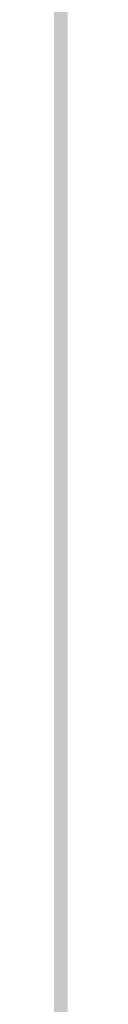
# Model space of a CAD drawing. Units: inches. Extents: x 2083 to 3317, y 1141 to 2115.
# Tile 192 of 256: x 3126.9582 to 3126.9594, y 1263.3548 to 1263.6134. Entities that reach past the tile are written whole.
import ezdxf

# ---------------------------------------------------------------- set-up
doc = ezdxf.new("R2010")
doc.units = ezdxf.units.IN
doc.layers.add('A-ANNO-DIMS', color=2, linetype='Continuous', lineweight=18)
doc.layers.add('A-WALL-PATT', color=251, linetype='Continuous', lineweight=13, true_color=0x636466)
doc.styles.get("Standard").update_dxf_attribs({"font": 'arial.ttf'})
doc.dimstyles.new('ISO-25', dxfattribs={"dimtxt": 12, "dimasz": 12, "dimexe": 1.25, "dimexo": 0.625, "dimtad": 1, "dimlunit": 3, "dimtxsty": 'Standard', "dimcen": 2.5, "dimadec": 0, "dimazin": 0, "dimtfac": 1, "dimtmove": 0, "dimatfit": 3, "dimfxl": 1, "dimarcsym": 0})

# ---------------------------------------------------------------- blocks, each defined once
blk = doc.blocks.new('*D26')
at = {"layer": 'A-ANNO-DIMS', "color": 0, "lineweight": -2, "transparency": 16777216}
for p, q in [((3088.98584, 1274.91509), (3088.98584, 1270.95196)), ((3111.24004, 1274.91509), (3111.24004, 1270.95196)), ((3076.98584, 1272.20196), (2840.26245, 1272.20196)), ((3111.24004, 1272.20196), (3088.98584, 1272.20196)), ((3123.24004, 1272.20196), (3135.24004, 1272.20196))]:
    blk.add_line(p, q, dxfattribs=at)
at = {"layer": 'A-ANNO-DIMS', "color": 0, "transparency": 16777216}
for points in [[(3076.98584, 1274.20196), (3076.98584, 1270.20196), (3088.98584, 1272.20196)], [(3123.24004, 1274.20196), (3123.24004, 1270.20196), (3111.24004, 1272.20196)]]:
    blk.add_solid(points, dxfattribs=at)
at = {"layer": 'Defpoints', "color": 0, "transparency": 16777216}
for p in [(3088.98584, 1275.54009), (3111.24004, 1275.54009), (3088.98584, 1272.20196)]:
    blk.add_point(p, dxfattribs=at)
at = {"layer": 'A-ANNO-DIMS', "color": 0, "transparency": 16777216, "insert": (2952.62415, 1279.0316), "char_height": 12, "attachment_point": 5}
blk.add_mtext('NIGHTSTAND 1\'-10 1/2" TYP.', dxfattribs=at)
blk = doc.blocks.new('*D27')
at = {"layer": 'A-ANNO-DIMS', "color": 0, "lineweight": -2, "transparency": 16777216}
for p, q in [((3114.57817, 1309.79428), (3114.57817, 1321.79428)), ((3111.86504, 1297.79428), (3115.82817, 1297.79428)), ((3114.57817, 1297.79428), (3114.57817, 1275.54009)), ((3111.86504, 1275.54009), (3115.82817, 1275.54009)), ((3114.57817, 1263.54009), (3114.57817, 1140.98859))]:
    blk.add_line(p, q, dxfattribs=at)
at = {"layer": 'A-ANNO-DIMS', "color": 0, "transparency": 16777216}
for points in [[(3112.57817, 1309.79428), (3116.57817, 1309.79428), (3114.57817, 1297.79428)], [(3112.57817, 1263.54009), (3116.57817, 1263.54009), (3114.57817, 1275.54009)]]:
    blk.add_solid(points, dxfattribs=at)
at = {"layer": 'Defpoints', "color": 0, "transparency": 16777216}
for p in [(3111.24004, 1297.79428), (3111.24004, 1275.54009), (3114.57817, 1275.54009)]:
    blk.add_point(p, dxfattribs=at)
at = {"layer": 'A-ANNO-DIMS', "color": 0, "transparency": 16777216, "insert": (3107.74853, 1196.26434), "char_height": 12, "attachment_point": 5, "rotation": 90}
blk.add_mtext('1\'-10 1/2" TYP.', dxfattribs=at)

msp = doc.modelspace()

# ---------------------------------------------------------------- hatches: boundary and pattern name
at = {"layer": 'A-WALL-PATT'}
h = msp.add_hatch(color=256, dxfattribs=at)
h.dxf.hatch_style = 1
h.paths.add_polyline_path([(3126.95978, 2020.76136), (2748.95978, 2020.76136), (2604.95978, 2020.76136), (2226.95978, 2020.76136), (2226.95978, 1702.76136), (2466.95978, 1702.76136), (2466.95978, 1582.76136), (2418.95978, 1582.76136), (2418.95978, 1477.76136), (2226.95978, 1477.76136), (2226.95978, 1263.26136), (2544.95978, 1263.26136), (2544.95978, 1411.76136), (2604.95978, 1411.76136), (2685.95978, 1411.76136), (2685.95978, 1420.76136), (2604.95978, 1420.76136), (2604.95978, 1573.76136), (2604.95978, 1702.76136), (2604.95978, 2011.76136), (2748.95978, 2011.76136), (2748.95978, 1702.76136), (2862.95978, 1702.76136), (2862.95978, 1621.76136), (2871.95978, 1621.76136), (2871.95978, 1702.76136), (2883.95978, 1702.76136), (2883.95978, 1706.93946, -0.026459), (2883.95978, 1711.76136), (2757.95978, 1711.76136), (2757.95978, 1807.76136), (2787.95978, 1807.76136), (2787.95978, 1812.26136), (2757.95978, 1812.26136), (2757.95978, 2011.76136), (2877.95978, 2011.76136), (2877.95978, 1812.26136), (2847.95978, 1812.26136), (2847.95978, 1807.76136), (2889.83574, 1807.76136), (2889.83574, 1812.26136), (2882.45978, 1812.26136), (2882.45978, 2011.76136), (3117.95978, 2011.76136), (3117.95978, 1812.26136), (2937.83574, 1812.26136), (2937.83574, 1807.76136), (2995.70978, 1807.76136), (2995.70978, 1796.11767), (3000.20978, 1796.11767), (3000.20978, 1807.76136), (3117.95978, 1807.76136), (3117.95978, 1711.76136), (3000.20978, 1711.76136), (3000.20978, 1760.11767), (2998.5727, 1760.11767, -0.020711), (2995.70978, 1760.11767), (2995.70978, 1711.76136), (2931.95978, 1711.76136), (2931.95978, 1702.76136), (3126.95978, 1702.76136)])
h.paths.add_polyline_path([(2471.45978, 2011.76136), (2471.45978, 1810.01136), (2462.71694, 1810.01136), (2462.71694, 1805.51136), (2505.95978, 1805.51136), (2505.95978, 1810.01136), (2475.95978, 1810.01136), (2475.95978, 2011.76136), (2595.95978, 2011.76136), (2595.95978, 1810.01136), (2565.95978, 1810.01136), (2565.95978, 1805.51136), (2595.95978, 1805.51136), (2595.95978, 1711.76136), (2235.95978, 1711.76136), (2235.95978, 1805.51136), (2353.70978, 1805.51136), (2353.70978, 1796.05416), (2358.20978, 1796.05416), (2358.20978, 1805.51136), (2414.71694, 1805.51136), (2414.71694, 1810.01136), (2235.95978, 1810.01136), (2235.95978, 2011.76136)], flags=16)
h.paths.add_polyline_path([(2270.20473, 1994.61001), (2270.20473, 1970.61001), (2246.20473, 1970.61001), (2246.20473, 1994.61001)], flags=0)
edge = h.paths.add_edge_path(flags=0)
edge.add_ellipse((2332.02739, 1899.79818), major_axis=(-3.04299, 3.04299), ratio=0.1682525, start_angle=-161.33217, end_angle=-156.30711, ccw=False)
edge.add_ellipse((2333.08204, 1898.74353), major_axis=(-1.05465, 1.05465), ratio=0.4535321, start_angle=-123.37102, end_angle=-94.15911)
edge = h.paths.add_edge_path(flags=0)
edge.add_ellipse((2332.02739, 1968.87629), major_axis=(3.04299, 3.04299), ratio=0.1682525, start_angle=18.66783, end_angle=23.69289)
edge.add_spline(control_points=[(2332.9256, 1970.6911), (2332.22677, 1970.3361), (2330.89371, 1969.65891), (2328.41308, 1970.93214), (2327.20393, 1967.74871), (2324.7096, 1969.95559), (2322.53282, 1967.01235), (2320.01285, 1971.29581), (2317.68031, 1968.15784), (2316.04053, 1967.10205), (2315.4269, 1966.8096)], knot_values=[0, 0, 0, 0, 2.267059, 4.324559, 6.685584, 8.878641, 11.121502, 14.300359, 17.755284, 19.732645, 19.732645, 19.732645, 19.732645], degree=3, periodic=0)
edge.add_ellipse((2332.02739, 1968.87629), major_axis=(3.04299, 3.04299), ratio=0.1682525, start_angle=18.66783, end_angle=23.69289, ccw=False)
edge.add_ellipse((2333.08204, 1969.93094), major_axis=(1.05465, 1.05465), ratio=0.4535321, start_angle=56.62898, end_angle=85.84089, ccw=False)
edge = h.paths.add_edge_path(flags=0)
edge.add_spline(control_points=[(2296.42829, 1967.98791), (2293.6278, 1965.33631), (2287.70362, 1959.72709), (2299.74386, 1949.9957), (2294.53259, 1935.66853), (2290.57323, 1920.60351), (2293.39412, 1909.97369), (2296.18541, 1904.96654)], knot_values=[0.099185, 0.099185, 0.099185, 0.099185, 0.345301, 0.619822, 0.982653, 1.386093, 1.810555, 1.810555, 1.810555, 1.810555], degree=3, periodic=0)
edge.add_spline(control_points=[(2296.18541, 1904.96654), (2297.38358, 1902.6193), (2298.00097, 1901.94931), (2298.55297, 1901.46815)], knot_values=[0.006246, 0.006246, 0.006246, 0.006246, 0.055476, 0.055476, 0.055476, 0.055476], degree=3, periodic=0)
edge.add_spline(control_points=[(2298.55297, 1901.46815), (2297.25861, 1900.92322), (2295.22529, 1900.23213), (2293.06023, 1900.61421), (2292.10142, 1900.78841), (2292.08958, 1900.79057)], knot_values=[0.312835, 0.312835, 0.312835, 0.312835, 0.40178, 0.474987, 0.475903, 0.475903, 0.475903, 0.475903], degree=3, periodic=0)
edge.add_arc((2292.79365, 1904.66411), 3.93701, 215.4209, 259.69818, ccw=False)
edge.add_spline(control_points=[(2289.58531, 1902.3823), (2289.47665, 1902.53509), (2289.36848, 1902.68804), (2289.26086, 1902.84117)], knot_values=[0.102872, 0.102872, 0.102872, 0.102872, 0.116896, 0.116896, 0.116896, 0.116896], degree=3, periodic=0)
edge.add_spline(control_points=[(2289.26086, 1902.84117), (2288.6866, 1902.55019), (2287.64005, 1902.0199), (2285.88134, 1901.87395), (2283.85297, 1901.50435), (2281.71999, 1899.71054), (2278.46699, 1899.49294), (2276.15714, 1901.8832), (2272.25895, 1899.80407), (2267.77761, 1901.84318), (2262.24388, 1900.18403), (2257.41493, 1901.78206), (2254.31837, 1900.72612), (2253.17828, 1900.33734)], knot_values=[0, 0, 0, 0, 1.907977, 3.477176, 5.261074, 7.972851, 11.680248, 13.717921, 16.939592, 22.789562, 27.502503, 33.595215, 37.145618, 37.145618, 37.145618, 37.145618], degree=3, periodic=0)
edge.add_line((2253.17828, 1900.33734), (2250.24424, 1902.84117))
edge.add_line((2250.24424, 1902.84117), (2250.24424, 1965.8333))
edge.add_line((2250.24424, 1965.8333), (2253.17828, 1968.33712))
edge.add_spline(control_points=[(2253.17828, 1968.33712), (2254.31837, 1967.94835), (2257.41493, 1966.89241), (2262.24388, 1968.49043), (2267.77761, 1966.83128), (2271.52673, 1968.53722), (2273.87591, 1967.82829), (2274.2067, 1967.72764)], knot_values=[0, 0, 0, 0, 0.09018, 0.244935, 0.364644, 0.513233, 0.537855, 0.537855, 0.537855, 0.537855], degree=3, periodic=0)
edge.add_arc((2274.35289, 1963.79335), 3.93701, 72.05113, 92.12795, ccw=False)
edge.add_arc((2281.29693, 1985.23), 18.5963, 252.051134, 288.565722)
edge.add_arc((2292.31672, 1956.02888), 12.64608, 71.026788, 113.778218, ccw=False)
edge = h.paths.add_edge_path(flags=0)
edge.add_spline(control_points=[(2274.89941, 1951.85619), (2275.06616, 1951.61659), (2275.23269, 1951.37659), (2275.39799, 1951.13585)], knot_values=[1.409916, 1.409916, 1.409916, 1.409916, 1.43159, 1.43159, 1.43159, 1.43159], degree=3, periodic=0)
edge.add_spline(control_points=[(2275.39799, 1951.13585), (2275.79211, 1950.56189), (2276.17923, 1949.98377), (2276.54555, 1949.3971)], knot_values=[1.358238, 1.358238, 1.358238, 1.358238, 1.409916, 1.409916, 1.409916, 1.409916], degree=3, periodic=0)
edge.add_line((2276.54555, 1949.3971), (2277.43729, 1947.86218))
edge.add_spline(control_points=[(2277.43729, 1947.86218), (2276.30383, 1945.67311), (2274.6397, 1942.42688), (2274.63161, 1938.0939), (2272.79912, 1930.85155), (2274.35643, 1943.89705), (2275.94768, 1947.92336), (2276.54555, 1949.3971)], knot_values=[0.005632, 0.005632, 0.005632, 0.005632, 0.186014, 0.266002, 0.357087, 0.59639, 0.739732, 0.739732, 0.739732, 0.739732], degree=3, periodic=0)
edge.add_spline(control_points=[(2276.54555, 1949.3971), (2276.17923, 1949.98377), (2275.79211, 1950.56189), (2275.39799, 1951.13585)], knot_values=[1.358238, 1.358238, 1.358238, 1.358238, 1.409916, 1.409916, 1.409916, 1.409916], degree=3, periodic=0)
edge.add_spline(control_points=[(2275.39799, 1951.13585), (2274.9425, 1950.08045), (2274.20776, 1948.02527), (2273.9346, 1944.85148), (2272.46853, 1937.62749), (2273.46622, 1945.69647), (2274.70062, 1951.05947), (2274.89941, 1951.85619)], knot_values=[0.104364, 0.104364, 0.104364, 0.104364, 0.189636, 0.269624, 0.36071, 0.600013, 0.644622, 0.644622, 0.644622, 0.644622], degree=3, periodic=0)
h.paths.add_polyline_path([(2269.16751, 1963.12757, -0.357527), (2268.17063, 1960.97637, -0.092561), (2268.17063, 1939.43632, -0.357527), (2269.16751, 1937.28512, -0.357527), (2267.01631, 1938.282, -0.164785), (2254.68558, 1938.282, -0.357527), (2252.53438, 1937.28512, -0.357527), (2253.53126, 1939.43632, -0.092561), (2253.53126, 1960.97637, -0.357527), (2252.53438, 1963.12757, -0.357527), (2254.68558, 1962.13069, -0.164785), (2267.01631, 1962.13069, -0.357527)], flags=0)
h.paths.add_polyline_path([(2248.87407, 1967.8018), (2248.87407, 1957.02771), (2249.45778, 1957.02771), (2249.45778, 1911.64676), (2248.87407, 1911.64676), (2248.87407, 1900.87267), (2246.51186, 1900.87267, 0.197327), (2244.14966, 1902.45687), (2244.14966, 1966.21759, 0.197327), (2246.51186, 1967.8018)], flags=0)
h.paths.add_polyline_path([(2269.16751, 1931.38934, -0.357527), (2268.17063, 1929.23814, -0.092561), (2268.17063, 1907.6981, -0.357527), (2269.16751, 1905.54689, -0.357527), (2267.01631, 1906.54377, -0.164785), (2254.68558, 1906.54377, -0.357527), (2252.53438, 1905.54689, -0.357527), (2253.53126, 1907.6981, -0.092561), (2253.53126, 1929.23814, -0.357527), (2252.53438, 1931.38934, -0.357527), (2254.68558, 1930.39246, -0.164785), (2267.01631, 1930.39246, -0.357527)], flags=0)
edge = h.paths.add_edge_path(flags=0)
edge.add_spline(control_points=[(2276.19686, 1906.7237), (2276.16814, 1909.02893), (2276.11405, 1913.37185), (2270.59842, 1924.92498), (2273.90517, 1919.01278), (2275.92171, 1916.26206), (2275.47457, 1912.40215), (2277.25787, 1910.38062), (2276.69604, 1908.22504), (2276.64622, 1906.81302), (2276.61782, 1906.00841)], knot_values=[0, 0, 0, 0, 8.61026, 16.221274, 18.843057, 23.804898, 27.440828, 29.356102, 31.203478, 33.650687, 33.650687, 33.650687, 33.650687], degree=3, periodic=0)
edge.add_spline(control_points=[(2276.61782, 1906.00841), (2276.62331, 1905.62414), (2276.49774, 1904.62866), (2275.44178, 1903.85473), (2274.93731, 1903.08045), (2274.85908, 1902.84117)], knot_values=[0.156488, 0.156488, 0.156488, 0.156488, 0.184398, 0.231376, 0.250598, 0.250598, 0.250598, 0.250598], degree=3, periodic=0)
edge.add_line((2274.85908, 1902.84117), (2276.50598, 1902.84117))
edge.add_spline(control_points=[(2276.50598, 1902.84117), (2276.78831, 1903.08494), (2277.66507, 1904.1252), (2278.24954, 1904.34074), (2277.65387, 1908.52739), (2278.15567, 1906.22781), (2278.10046, 1905.28595), (2278.84667, 1904.06901), (2277.85679, 1903.41495), (2277.87419, 1902.99105), (2277.90356, 1902.84117)], knot_values=[0.059574, 0.059574, 0.059574, 0.059574, 0.080753, 0.103741, 0.16972, 0.176036, 0.207137, 0.240474, 0.262341, 0.27366, 0.27366, 0.27366, 0.27366], degree=3, periodic=0)
edge.add_line((2277.90356, 1902.84117), (2280.02983, 1902.84117))
edge.add_spline(control_points=[(2280.02983, 1902.84117), (2279.88822, 1903.0884), (2279.49926, 1903.98155), (2280.15228, 1905.93935), (2278.10362, 1909.65776), (2279.76239, 1907.18529), (2280.3279, 1904.87486), (2280.48511, 1903.48959), (2281.46327, 1903.24943), (2281.75834, 1902.9365), (2281.83404, 1902.84117)], knot_values=[0.013856, 0.013856, 0.013856, 0.013856, 0.034874, 0.088867, 0.107879, 0.126738, 0.158714, 0.193757, 0.217487, 0.226722, 0.226722, 0.226722, 0.226722], degree=3, periodic=0)
edge.add_spline(control_points=[(2281.83404, 1902.84117), (2281.78753, 1902.8267), (2281.64702, 1902.78299), (2281.39553, 1902.85949), (2281.08808, 1902.98524), (2280.72068, 1903.0609), (2280.33345, 1903.02573), (2280.12477, 1902.89888), (2280.02983, 1902.84117)], knot_values=[0, 0, 0, 0, 0.14413, 0.435517, 0.749276, 1.153046, 1.548371, 1.878348, 1.878348, 1.878348, 1.878348], degree=3, periodic=0)
edge.add_line((2280.02983, 1902.84117), (2277.90356, 1902.84117))
edge.add_spline(control_points=[(2277.90356, 1902.84117), (2277.89286, 1902.79586), (2277.8654, 1902.67964), (2277.60748, 1902.68748), (2277.27405, 1902.8007), (2276.83792, 1902.61977), (2276.58381, 1902.78926), (2276.50598, 1902.84117)], knot_values=[0, 0, 0, 0, 0.127189, 0.326199, 0.628009, 1.24357, 1.515331, 1.515331, 1.515331, 1.515331], degree=3, periodic=0)
edge.add_line((2276.50598, 1902.84117), (2274.85908, 1902.84117))
edge.add_spline(control_points=[(2274.85908, 1902.84117), (2274.81444, 1902.89859), (2274.72513, 1903.01345), (2274.49348, 1903.11897), (2274.24429, 1902.96054), (2273.93712, 1903.18494), (2273.61404, 1902.98314), (2273.40832, 1902.88304), (2273.32225, 1902.84117)], knot_values=[0, 0, 0, 0, 0.21843, 0.436957, 0.687977, 0.990379, 1.398396, 1.69185, 1.69185, 1.69185, 1.69185], degree=3, periodic=0)
edge.add_spline(control_points=[(2273.32225, 1902.84117), (2273.61674, 1903.44569), (2274.274, 1904.53825), (2276.02724, 1904.5737), (2276.20696, 1906.58364), (2276.19686, 1906.7237)], knot_values=[0.012227, 0.012227, 0.012227, 0.012227, 0.059472, 0.106218, 0.134458, 0.134458, 0.134458, 0.134458], degree=3, periodic=0)
h.paths.add_polyline_path([(2270.77605, 1897.78983), (2270.77605, 1873.78983), (2246.77605, 1873.78983), (2246.77605, 1897.78983)], flags=0)
h.paths.add_polyline_path([(2353.70978, 1760.00506), (2353.70978, 1760.05416), (2358.20978, 1760.05416, -0.033729)], flags=0)
h.paths.add_polyline_path([(2321.81912, 1737.52919), (2341.99533, 1737.52919, -0.414214), (2343.20327, 1736.32124), (2343.20327, 1721.0206, -0.414214), (2341.99533, 1719.81265), (2321.81912, 1719.81265, -0.414214), (2320.61117, 1721.0206), (2320.61117, 1736.32124, -0.414214)], flags=0)
h.paths.add_polyline_path([(2324.23501, 1736.32124), (2339.57944, 1736.32124, -0.414214), (2341.99533, 1733.90535), (2341.99533, 1725.44973, -0.414214), (2339.57944, 1723.03384), (2333.68059, 1723.03384), (2333.84532, 1722.04547, -0.870646), (2335.4254, 1721.82589, -0.767327), (2333.92269, 1721.42324), (2331.29102, 1721.42324, -0.767327), (2329.78832, 1721.82589, -0.870646), (2331.3684, 1722.04547), (2331.53313, 1723.03384), (2324.23501, 1723.03384, -0.414214), (2321.81912, 1725.44973), (2321.81912, 1733.90535, -0.414214)], flags=0)
h.paths.add_polyline_path([(2570.48379, 1928.61544), (2589.68379, 1928.61544), (2590.16883, 1928.61544), (2590.16883, 1904.9934), (2570.48379, 1904.9934)], flags=0)
h.paths.add_polyline_path([(2574.44732, 1927.26382, -1), (2572.82884, 1927.26382, -1)], flags=0)
h.paths.add_polyline_path([(2573.08987, 1926.94088), (2573.92503, 1927.77604), (2574.14774, 1927.55333), (2573.31258, 1926.71817)], flags=0)
h.paths.add_polyline_path([(2578.77906, 1919.72962, -1), (2571.59166, 1919.72962, -1)], flags=0)
h.paths.add_polyline_path([(2578.38536, 1919.72962, -1), (2571.98536, 1919.72962, -1)], flags=0)
h.paths.add_polyline_path([(2331.59576, 1729.47622, -1), (2333.61795, 1729.47622, -1)], flags=0)
h.paths.add_polyline_path([(2578.03423, 1927.26382, -1), (2576.41574, 1927.26382, -1)], flags=0)
h.paths.add_polyline_path([(2576.68885, 1927.53109), (2576.91156, 1927.7538), (2577.74673, 1926.91863), (2577.52402, 1926.69592)], flags=0)
h.paths.add_polyline_path([(2578.13906, 1909.85954, -1), (2572.23166, 1909.85954, -1)], flags=0)
h.paths.add_polyline_path([(2577.74536, 1909.85954, -1), (2572.62536, 1909.85954, -1)], flags=0)
h.paths.add_polyline_path([(2583.79772, 1927.26382, -1), (2582.17923, 1927.26382, -1)], flags=0)
h.paths.add_polyline_path([(2582.71865, 1927.7538), (2583.55381, 1926.91863), (2583.3311, 1926.69592), (2582.49594, 1927.53109)], flags=0)
h.paths.add_polyline_path([(2582.49594, 1927.53109), (2582.71865, 1927.7538), (2583.55381, 1926.91863), (2583.3311, 1926.69592)], flags=0)
h.paths.add_polyline_path([(2587.73906, 1920.52962, -1), (2581.83166, 1920.52962, -1)], flags=0)
h.paths.add_polyline_path([(2587.34536, 1920.52962, -1), (2582.22536, 1920.52962, -1)], flags=0)
h.paths.add_polyline_path([(2587.38462, 1927.26382, -1), (2585.76613, 1927.26382, -1)], flags=0)
h.paths.add_polyline_path([(2586.08199, 1926.98025), (2586.91716, 1927.81541), (2587.13987, 1927.5927), (2586.3047, 1926.75754)], flags=0)
h.paths.add_polyline_path([(2588.37906, 1910.65954, -1), (2581.19166, 1910.65954, -1)], flags=0)
h.paths.add_polyline_path([(2587.98536, 1910.65954, -1), (2581.58536, 1910.65954, -1)], flags=0)
h.paths.add_polyline_path([(2417.16773, 1729.4779), (2437.34394, 1729.4779, -0.414214), (2438.55188, 1728.26995), (2438.55188, 1712.96931, -0.414214), (2437.34394, 1711.76136), (2417.16773, 1711.76136, -0.414214), (2415.95978, 1712.96931), (2415.95978, 1728.26995, -0.414214)], flags=0)
h.paths.add_polyline_path([(2419.58362, 1728.26995), (2434.92805, 1728.26995, -0.414214), (2437.34394, 1725.85406), (2437.34394, 1717.39844, -0.414214), (2434.92805, 1714.98255), (2429.0292, 1714.98255), (2429.19393, 1713.99418, -0.870646), (2430.77401, 1713.7746, -0.767327), (2429.2713, 1713.37195), (2426.63963, 1713.37195, -0.767327), (2425.13693, 1713.7746, -0.870646), (2426.71701, 1713.99418), (2426.88174, 1714.98255), (2419.58362, 1714.98255, -0.414214), (2417.16773, 1717.39844), (2417.16773, 1725.85406, -0.414214)], flags=0)
h.paths.add_polyline_path([(2419.58362, 1728.26995), (2434.92805, 1728.26995, -0.414214), (2437.34394, 1725.85406), (2437.34394, 1717.39844, -0.414214), (2434.92805, 1714.98255), (2429.0292, 1714.98255), (2428.35812, 1719.00903), (2427.55282, 1719.00903), (2426.88174, 1714.98255), (2419.58362, 1714.98255, -0.414214), (2417.16773, 1717.39844), (2417.16773, 1725.85406, -0.414214)], flags=0)
h.paths.add_polyline_path([(2426.94437, 1721.42492, -1), (2428.96656, 1721.42492, -1)], flags=0)
h.paths.add_polyline_path([(2475.95978, 1702.76136), (2595.95978, 1702.76136), (2595.95978, 1582.76136), (2475.95978, 1582.76136)], flags=16)
h.paths.add_polyline_path([(2427.95978, 1573.76136), (2595.95978, 1573.76136), (2595.95978, 1468.76136), (2595.95978, 1420.76136), (2384.45978, 1420.76136), (2384.45978, 1468.76136), (2427.95978, 1468.76136)], flags=16)
h.paths.add_polyline_path([(2379.95978, 1468.76136), (2379.95978, 1420.76136), (2235.95978, 1420.76136), (2235.95978, 1468.76136)], flags=16)
h.paths.add_polyline_path([(2317.816, 1466.69577), (2337.9922, 1466.69577, -0.414214), (2339.20015, 1465.48782), (2339.20015, 1450.18718, -0.414214), (2337.9922, 1448.97923), (2317.816, 1448.97923, -0.414214), (2316.60805, 1450.18718), (2316.60805, 1465.48782, -0.414214)], flags=0)
h.paths.add_polyline_path([(2320.23189, 1465.48782), (2335.57631, 1465.48782, -0.414214), (2337.9922, 1463.07193), (2337.9922, 1454.61631, -0.414214), (2335.57631, 1452.20042), (2329.67747, 1452.20042), (2329.84219, 1451.21205, -0.870646), (2331.42228, 1450.99247, -0.767327), (2329.91957, 1450.58983), (2327.2879, 1450.58983, -0.767327), (2325.7852, 1450.99247, -0.870646), (2327.36528, 1451.21205), (2327.53001, 1452.20042), (2320.23189, 1452.20042, -0.414214), (2317.816, 1454.61631), (2317.816, 1463.07193, -0.414214)], flags=0)
h.paths.add_polyline_path([(2320.23189, 1465.48782), (2335.57631, 1465.48782, -0.414214), (2337.9922, 1463.07193), (2337.9922, 1454.61631, -0.414214), (2335.57631, 1452.20042), (2329.67747, 1452.20042), (2329.00638, 1456.22691), (2328.20109, 1456.22691), (2327.53001, 1452.20042), (2320.23189, 1452.20042, -0.414214), (2317.816, 1454.61631), (2317.816, 1463.07193, -0.414214)], flags=0)
h.paths.add_polyline_path([(2327.59264, 1458.6428, -1), (2329.61483, 1458.6428, -1)], flags=0)
h.paths.add_polyline_path([(2244.41174, 1433.34045), (2241.92094, 1433.34045, -0.414214), (2240.01786, 1435.24354), (2240.01786, 1440.95281, -0.414211), (2241.92093, 1442.8559), (2244.41174, 1442.8559, -1.976472)], flags=0)
h.paths.add_polyline_path([(2245.35689, 1434.39754, -0.414214), (2245.35689, 1441.79881, -2.144098)], flags=0)
h.paths.add_polyline_path([(2535.95978, 1416.26136), (2535.95978, 1272.26136), (2235.95978, 1272.26136), (2235.95978, 1416.26136)], flags=16)
h.paths.add_polyline_path([(2260.11956, 1384.29284), (2260.11956, 1362.03865), (2237.86537, 1362.03865), (2237.86537, 1384.29284)], flags=0)
edge = h.paths.add_edge_path(flags=0)
edge.add_line((2318.25185, 1362.0933), (2318.1458, 1362.00097))
edge.add_ellipse((2317.44512, 1360.43104), major_axis=(2.82164, 2.82164), ratio=0.1682525, start_angle=18.66783, end_angle=20.94813, ccw=False)
edge.add_ellipse((2318.42305, 1361.40897), major_axis=(0.97793, 0.97793), ratio=0.4535321, start_angle=56.62898, end_angle=70.2262, ccw=False)
edge = h.paths.add_edge_path(flags=0)
edge.add_line((2319.10737, 1295.57108), (2319.01504, 1295.67713))
edge.add_ellipse((2317.44512, 1296.37781), major_axis=(-2.82164, 2.82164), ratio=0.1682525, start_angle=-161.33217, end_angle=-159.05187, ccw=False)
edge.add_ellipse((2318.42305, 1295.39988), major_axis=(-0.97793, 0.97793), ratio=0.4535321, start_angle=-123.37102, end_angle=-109.7738)
edge = h.paths.add_edge_path(flags=0)
edge.add_spline(control_points=[(2284.21035, 1301.17022), (2284.58069, 1300.44472), (2284.89119, 1299.89202), (2285.15955, 1299.46102)], knot_values=[0.039066, 0.039066, 0.039066, 0.039066, 0.055476, 0.055476, 0.055476, 0.055476], degree=3, periodic=0)
edge.add_line((2285.15955, 1299.46102), (2284.21035, 1301.17022))
edge = h.paths.add_edge_path(flags=0)
edge.add_line((2280.41246, 1297.29801), (2283.36999, 1297.03612))
edge.add_line((2283.36999, 1297.03612), (2286.40569, 1297.92631))
edge.add_spline(control_points=[(2286.40569, 1297.92631), (2285.30549, 1297.46312), (2284.34478, 1297.12915), (2283.36999, 1297.03612)], knot_values=[0.394369, 0.394369, 0.394369, 0.394369, 0.475903, 0.475903, 0.475903, 0.475903], degree=3, periodic=0)
edge.add_spline(control_points=[(2283.36999, 1297.03612), (2283.28139, 1297.02767), (2282.31629, 1296.95734), (2281.3125, 1297.13448), (2280.42344, 1297.29602), (2280.41246, 1297.29801)], knot_values=[0.312835, 0.312835, 0.312835, 0.312835, 0.320246, 0.393453, 0.394369, 0.394369, 0.394369, 0.394369], degree=3, periodic=0)
edge = h.paths.add_edge_path(flags=0)
edge.add_line((2284.43556, 1359.60729), (2280.44629, 1355.32805))
edge.add_line((2280.44629, 1355.32805), (2279.57999, 1351.01775))
edge.add_line((2279.57999, 1351.01775), (2282.41297, 1346.58043))
edge.add_spline(control_points=[(2282.41297, 1346.58043), (2283.15333, 1345.58924), (2284.2529, 1344.0289), (2284.80104, 1342.38717), (2284.93516, 1341.80554)], knot_values=[1.240098, 1.240098, 1.240098, 1.240098, 1.332892, 1.382712, 1.382712, 1.382712, 1.382712], degree=3, periodic=0)
edge.add_spline(control_points=[(2284.93516, 1341.80554), (2285.31911, 1340.1406), (2285.23303, 1338.4092), (2284.90994, 1336.65412)], knot_values=[1.097484, 1.097484, 1.097484, 1.097484, 1.240098, 1.240098, 1.240098, 1.240098], degree=3, periodic=0)
edge.add_spline(control_points=[(2284.90994, 1336.65412), (2284.58685, 1334.89904), (2284.02675, 1333.12027), (2283.46264, 1331.36058)], knot_values=[0.95487, 0.95487, 0.95487, 0.95487, 1.097484, 1.097484, 1.097484, 1.097484], degree=3, periodic=0)
edge.add_line((2283.46264, 1331.36058), (2281.89038, 1326.15336))
edge.add_line((2281.89038, 1326.15336), (2280.75626, 1321.05609))
edge.add_line((2280.75626, 1321.05609), (2280.2992, 1316.00198))
edge.add_line((2280.2992, 1316.00198), (2280.71593, 1310.95007))
edge.add_line((2280.71593, 1310.95007), (2282.02809, 1305.97214))
edge.add_line((2282.02809, 1305.97214), (2284.21035, 1301.17022))
edge.add_spline(control_points=[(2284.21035, 1301.17022), (2283.34073, 1302.73019), (2282.6119, 1304.33649), (2282.02809, 1305.97214)], knot_values=[0.099185, 0.099185, 0.099185, 0.099185, 0.241799, 0.241799, 0.241799, 0.241799], degree=3, periodic=0)
edge.add_spline(control_points=[(2282.02809, 1305.97214), (2281.44428, 1307.60778), (2281.00549, 1309.27276), (2280.71593, 1310.95007)], knot_values=[0.241799, 0.241799, 0.241799, 0.241799, 0.384413, 0.384413, 0.384413, 0.384413], degree=3, periodic=0)
edge.add_spline(control_points=[(2280.71593, 1310.95007), (2280.43324, 1312.58761), (2280.28939, 1314.27696), (2280.29889, 1315.96203), (2280.2992, 1316.00198)], knot_values=[0.384413, 0.384413, 0.384413, 0.384413, 0.523647, 0.527028, 0.527028, 0.527028, 0.527028], degree=3, periodic=0)
edge.add_spline(control_points=[(2280.2992, 1316.00198), (2280.31233, 1317.68696), (2280.47787, 1319.36793), (2280.75626, 1321.05609)], knot_values=[0.527028, 0.527028, 0.527028, 0.527028, 0.669642, 0.669642, 0.669642, 0.669642], degree=3, periodic=0)
edge.add_spline(control_points=[(2280.75626, 1321.05609), (2281.03465, 1322.74425), (2281.42588, 1324.43961), (2281.89038, 1326.15336)], knot_values=[0.669642, 0.669642, 0.669642, 0.669642, 0.812256, 0.812256, 0.812256, 0.812256], degree=3, periodic=0)
edge.add_spline(control_points=[(2281.89038, 1326.15336), (2282.26438, 1327.53325), (2282.78787, 1329.26181), (2283.35275, 1331.01778), (2283.46264, 1331.36058)], knot_values=[0.812256, 0.812256, 0.812256, 0.812256, 0.927087, 0.95487, 0.95487, 0.95487, 0.95487], degree=3, periodic=0)
edge.add_line((2283.46264, 1331.36058), (2284.90994, 1336.65412))
edge.add_line((2284.90994, 1336.65412), (2284.93516, 1341.80554))
edge.add_line((2284.93516, 1341.80554), (2282.41297, 1346.58043))
edge.add_spline(control_points=[(2282.41297, 1346.58043), (2281.27513, 1348.10379), (2280.07845, 1349.57032), (2279.57999, 1351.01775)], knot_values=[1.382712, 1.382712, 1.382712, 1.382712, 1.525326, 1.525326, 1.525326, 1.525326], degree=3, periodic=0)
edge.add_spline(control_points=[(2279.57999, 1351.01775), (2279.44328, 1351.41472), (2279.13631, 1352.85692), (2279.73519, 1354.29039), (2280.44629, 1355.32805)], knot_values=[1.525326, 1.525326, 1.525326, 1.525326, 1.564439, 1.667941, 1.667941, 1.667941, 1.667941], degree=3, periodic=0)
edge.add_spline(control_points=[(2280.44629, 1355.32805), (2281.42611, 1356.75784), (2282.93084, 1358.18256), (2284.43556, 1359.60729)], knot_values=[1.667941, 1.667941, 1.667941, 1.667941, 1.810555, 1.810555, 1.810555, 1.810555], degree=3, periodic=0)
edge.add_arc((2280.62307, 1348.51818), 11.72618, 71.026788, 113.778218)
edge.add_arc((2270.40489, 1375.59516), 17.24357, 252.051134, 288.565722, ccw=False)
edge.add_arc((2263.96597, 1355.71785), 3.65062, 72.05113, 92.12795)
edge.add_arc((2263.96597, 1355.71785), 3.65062, 92.12795, 177.98513)
edge.add_spline(control_points=[(2260.3176, 1355.8462), (2260.26042, 1354.22067), (2260.55128, 1350.18655), (2262.99934, 1346.76625), (2264.47274, 1344.64902)], knot_values=[1.43159, 1.43159, 1.43159, 1.43159, 1.564144, 1.770695, 1.770695, 1.770695, 1.770695], degree=3, periodic=0)
edge.add_line((2264.47274, 1344.64902), (2264.93559, 1343.98253))
edge.add_spline(control_points=[(2263.80104, 1340.24811), (2263.84324, 1340.51409), (2264.06724, 1341.75647), (2264.51269, 1343.00245), (2264.93505, 1343.98108)], knot_values=[0.53657, 0.53657, 0.53657, 0.53657, 0.559349, 0.644622, 0.644622, 0.644622, 0.644622], degree=3, periodic=0)
edge.add_spline(control_points=[(2264.93505, 1343.98108), (2265.11777, 1343.71497), (2265.29888, 1343.44791), (2265.47676, 1343.17936)], knot_values=[1.384077, 1.384077, 1.384077, 1.384077, 1.409916, 1.409916, 1.409916, 1.409916], degree=3, periodic=0)
edge.add_spline(control_points=[(2265.47676, 1343.17936), (2265.65464, 1342.91082), (2265.8293, 1342.64081), (2265.99913, 1342.36881)], knot_values=[1.358238, 1.358238, 1.358238, 1.358238, 1.384077, 1.384077, 1.384077, 1.384077], degree=3, periodic=0)
edge.add_line((2265.99913, 1342.36881), (2266.82601, 1340.94555))
edge.add_spline(control_points=[(2266.82601, 1340.94555), (2268.8944, 1337.08969), (2271.39817, 1325.843), (2270.51616, 1310.56856), (2275.91938, 1301.86061), (2277.78951, 1299.19945)], knot_values=[0.116896, 0.116896, 0.116896, 0.116896, 0.472987, 1.050969, 1.313793, 1.313793, 1.313793, 1.313793], degree=3, periodic=0)
edge.add_spline(control_points=[(2277.78951, 1299.19945), (2277.83941, 1299.12845), (2277.88943, 1299.0575), (2277.93957, 1298.98658)], knot_values=[0.109884, 0.109884, 0.109884, 0.109884, 0.116896, 0.116896, 0.116896, 0.116896], degree=3, periodic=0)
edge.add_line((2277.93957, 1298.98658), (2277.78885, 1299.19911))
edge.add_spline(control_points=[(2277.78885, 1299.19911), (2277.25658, 1298.92941), (2276.28635, 1298.4379), (2275.03935, 1298.33442), (2274.38333, 1298.2389), (2274.21525, 1298.20934)], knot_values=[33.12187, 33.12187, 33.12187, 33.12187, 35.029056, 36.598255, 37.144827, 37.144827, 37.144827, 37.144827], degree=3, periodic=0)
edge.add_line((2274.21525, 1298.20934), (2273.07315, 1297.89296))
edge.add_spline(control_points=[(2273.07315, 1297.89296), (2272.32294, 1297.57978), (2271.03915, 1296.51051), (2269.24839, 1296.22606), (2268.4231, 1296.37465)], knot_values=[26.532584, 26.532584, 26.532584, 26.532584, 29.198919, 31.839101, 31.839101, 31.839101, 31.839101], degree=3, periodic=0)
edge.add_line((2268.4231, 1296.37465), (2263.8785, 1297.45753))
edge.add_spline(control_points=[(2263.8785, 1297.45753), (2263.55608, 1297.35943), (2261.86031, 1296.83869), (2260.23878, 1297.28241), (2258.93345, 1297.51646)], knot_values=[15.919551, 15.919551, 15.919551, 15.919551, 16.939592, 21.226067, 21.226067, 21.226067, 21.226067], degree=3, periodic=0)
edge.add_line((2258.93345, 1297.51646), (2254.05523, 1297.32901))
edge.add_spline(control_points=[(2254.05523, 1297.32901), (2253.75553, 1297.29582), (2252.11368, 1297.16517), (2250.46187, 1297.54422), (2249.12969, 1297.66788)], knot_values=[5.306517, 5.306517, 5.306517, 5.306517, 6.276435, 10.613034, 10.613034, 10.613034, 10.613034], degree=3, periodic=0)
edge.add_line((2249.12969, 1297.66788), (2244.33165, 1296.87776))
edge.add_line((2244.33165, 1296.87776), (2241.61103, 1299.19945))
edge.add_line((2241.61103, 1299.19945), (2241.61103, 1357.6094))
edge.add_line((2241.61103, 1357.6094), (2244.33165, 1359.9311))
edge.add_line((2244.33165, 1359.9311), (2252.72882, 1359.54269))
edge.add_spline(control_points=[(2252.72882, 1359.54269), (2252.87094, 1359.54644), (2253.30574, 1359.54817), (2253.73984, 1359.51427), (2254.03174, 1359.48243)], knot_values=[0.233291, 0.233291, 0.233291, 0.233291, 0.244935, 0.268927, 0.268927, 0.268927, 0.268927], degree=3, periodic=0)
edge.add_line((2254.03174, 1359.48243), (2259.58719, 1359.41639))
edge.add_spline(control_points=[(2259.58719, 1359.41639), (2260.67707, 1359.6285), (2262.0732, 1359.897), (2263.52369, 1359.45928), (2263.83042, 1359.36595)], knot_values=[0.422516, 0.422516, 0.422516, 0.422516, 0.513233, 0.537855, 0.537855, 0.537855, 0.537855], degree=3, periodic=0)
edge.add_arc((2263.96597, 1355.71785), 3.65062, 72.05113, 92.12795, ccw=False)
edge.add_arc((2270.40489, 1375.59516), 17.24357, 252.051134, 288.565722)
edge.add_arc((2280.62307, 1348.51818), 11.72618, 71.026788, 113.778218, ccw=False)
h.paths.add_polyline_path([(2240.34053, 1359.43471), (2240.34053, 1349.44435), (2240.88178, 1349.44435), (2240.88178, 1307.3645), (2240.34053, 1307.3645), (2240.34053, 1297.37414), (2238.15016, 1297.37414, 0.197327), (2235.95978, 1298.84311), (2235.95978, 1357.96575, 0.197327), (2238.15016, 1359.43471)], flags=0)
h.paths.add_polyline_path([(2259.15779, 1355.1005, -0.357527), (2258.23342, 1353.10578, -0.092561), (2258.23342, 1333.1326, -0.357527), (2259.15779, 1331.13788, -0.357527), (2257.16307, 1332.06225, -0.164785), (2245.7293, 1332.06225, -0.357527), (2243.73458, 1331.13788, -0.357527), (2244.65895, 1333.1326, -0.092561), (2244.65895, 1353.10578, -0.357527), (2243.73458, 1355.1005, -0.357527), (2245.7293, 1354.17613, -0.164785), (2257.16307, 1354.17613, -0.357527)], flags=0)
edge = h.paths.add_edge_path(flags=0)
edge.add_line((2265.99913, 1342.36881), (2266.82601, 1340.94555))
edge.add_line((2266.82601, 1340.94555), (2265.30756, 1337.81407))
edge.add_line((2265.30756, 1337.81407), (2264.35823, 1334.65294))
edge.add_line((2264.35823, 1334.65294), (2264.26201, 1333.7997))
edge.add_spline(control_points=[(2264.26201, 1333.7997), (2264.20836, 1333.18705), (2264.16206, 1332.36553), (2264.00714, 1331.41393), (2263.96905, 1331.20183)], knot_values=[0.464444, 0.464444, 0.464444, 0.464444, 0.516691, 0.531608, 0.531608, 0.531608, 0.531608], degree=3, periodic=0)
edge.add_spline(control_points=[(2263.96905, 1331.20183), (2263.77453, 1330.11887), (2263.42437, 1328.79084), (2263.25742, 1328.53065), (2263.23403, 1328.51461)], knot_values=[0.372682, 0.372682, 0.372682, 0.372682, 0.44885, 0.464444, 0.464444, 0.464444, 0.464444], degree=3, periodic=0)
edge.add_spline(control_points=[(2263.23403, 1328.51461), (2263.09638, 1328.42023), (2263.13117, 1329.30148), (2263.27495, 1330.61575)], knot_values=[0.280919, 0.280919, 0.280919, 0.280919, 0.372682, 0.372682, 0.372682, 0.372682], degree=3, periodic=0)
edge.add_spline(control_points=[(2263.27495, 1330.61575), (2263.41874, 1331.93002), (2263.67152, 1333.67732), (2263.96985, 1335.31503)], knot_values=[0.189157, 0.189157, 0.189157, 0.189157, 0.280919, 0.280919, 0.280919, 0.280919], degree=3, periodic=0)
edge.add_spline(control_points=[(2263.96985, 1335.31503), (2264.1005, 1336.03219), (2264.41878, 1337.62191), (2264.75485, 1338.86443), (2264.94742, 1339.49112)], knot_values=[0.097394, 0.097394, 0.097394, 0.097394, 0.137578, 0.189157, 0.189157, 0.189157, 0.189157], degree=3, periodic=0)
edge.add_spline(control_points=[(2264.94742, 1339.49112), (2265.29002, 1340.60605), (2265.64424, 1341.494), (2265.99913, 1342.36881)], knot_values=[0.005632, 0.005632, 0.005632, 0.005632, 0.097394, 0.097394, 0.097394, 0.097394], degree=3, periodic=0)
h.paths.add_polyline_path([(2259.15779, 1325.67097, -0.357527), (2258.23342, 1323.67625, -0.092561), (2258.23342, 1303.70307, -0.357527), (2259.15779, 1301.70835, -0.357527), (2257.16307, 1302.63272, -0.164785), (2245.7293, 1302.63272, -0.357527), (2243.73458, 1301.70835, -0.357527), (2244.65895, 1303.70307, -0.092561), (2244.65895, 1323.67625, -0.357527), (2243.73458, 1325.67097, -0.357527), (2245.7293, 1324.74661, -0.164785), (2257.16307, 1324.74661, -0.357527)], flags=0)
edge = h.paths.add_edge_path(flags=0)
edge.add_spline(control_points=[(2261.70894, 1317.31142), (2261.67948, 1317.41758), (2261.76186, 1317.38853), (2262.49074, 1316.08987), (2262.96218, 1315.3009)], knot_values=[14.955861, 14.955861, 14.955861, 14.955861, 16.221274, 18.694826, 18.694826, 18.694826, 18.694826], degree=3, periodic=0)
edge.add_spline(control_points=[(2262.96218, 1315.3009), (2262.99044, 1315.25362), (2263.7021, 1314.06738), (2264.34898, 1313.12715), (2264.73005, 1312.16415)], knot_values=[18.694826, 18.694826, 18.694826, 18.694826, 18.843057, 22.433791, 22.433791, 22.433791, 22.433791], degree=3, periodic=0)
edge.add_spline(control_points=[(2264.73005, 1312.16415), (2264.87556, 1311.79644), (2265.17687, 1310.76981), (2265.14307, 1309.55926), (2265.24774, 1308.82419)], knot_values=[22.433791, 22.433791, 22.433791, 22.433791, 23.804898, 26.172756, 26.172756, 26.172756, 26.172756], degree=3, periodic=0)
edge.add_line((2265.24774, 1308.82419), (2265.85077, 1307.17189))
edge.add_spline(control_points=[(2265.85077, 1307.17189), (2266.06502, 1306.82168), (2266.38439, 1306.33225), (2266.4244, 1305.78055), (2266.42037, 1305.61122)], knot_values=[28.062562, 28.062562, 28.062562, 28.062562, 29.356102, 29.911721, 29.911721, 29.911721, 29.911721], degree=3, periodic=0)
edge.add_spline(control_points=[(2266.42037, 1305.61122), (2266.41612, 1305.43259), (2266.394, 1305.25), (2266.36478, 1305.06586)], knot_values=[29.911721, 29.911721, 29.911721, 29.911721, 30.497837, 30.497837, 30.497837, 30.497837], degree=3, periodic=0)
edge.add_line((2266.36478, 1305.06586), (2266.06615, 1302.1363))
edge.add_spline(control_points=[(2266.06615, 1302.1363), (2266.07124, 1301.77998), (2265.99808, 1301.19998), (2265.66327, 1300.75896), (2265.50891, 1300.58588)], knot_values=[0.156488, 0.156488, 0.156488, 0.156488, 0.184398, 0.203543, 0.203543, 0.203543, 0.203543], degree=3, periodic=0)
edge.add_line((2265.50891, 1300.58588), (2264.43534, 1299.19945))
edge.add_line((2264.43534, 1299.19945), (2265.96244, 1299.19945))
edge.add_line((2265.96244, 1299.19945), (2267.33599, 1301.17528))
edge.add_line((2267.33599, 1301.17528), (2267.31167, 1301.98624))
edge.add_spline(control_points=[(2267.31167, 1301.98624), (2267.26111, 1302.8624), (2267.16021, 1303.73713), (2267.27149, 1303.3259)], knot_values=[0.126229, 0.126229, 0.126229, 0.126229, 0.166617, 0.166617, 0.166617, 0.166617], degree=3, periodic=0)
edge.add_spline(control_points=[(2267.27149, 1303.3259), (2267.28003, 1303.2943), (2267.30979, 1303.17537), (2267.37345, 1302.88361), (2267.40612, 1302.68283), (2267.41793, 1302.60103)], knot_values=[0.166617, 0.166617, 0.166617, 0.166617, 0.16972, 0.176036, 0.180765, 0.180765, 0.180765, 0.180765], degree=3, periodic=0)
edge.add_spline(control_points=[(2267.74389, 1300.9875), (2267.68758, 1301.15094), (2267.48052, 1301.65666), (2267.48375, 1302.14479), (2267.41793, 1302.60103)], knot_values=[0.180765, 0.180765, 0.180765, 0.180765, 0.193767, 0.220139, 0.220139, 0.220139, 0.220139], degree=3, periodic=0)
edge.add_line((2267.41793, 1302.60103), (2267.74389, 1300.9875))
edge.add_spline(control_points=[(2267.74389, 1300.9875), (2267.83196, 1300.73188), (2267.93202, 1300.3099), (2267.55484, 1299.97452), (2267.42937, 1299.82921)], knot_values=[0.220139, 0.220139, 0.220139, 0.220139, 0.240474, 0.25489, 0.25489, 0.25489, 0.25489], degree=3, periodic=0)
edge.add_line((2267.42937, 1299.82921), (2267.25836, 1299.19945))
edge.add_line((2267.25836, 1299.19945), (2269.22996, 1299.19945))
edge.add_spline(control_points=[(2269.22996, 1299.19945), (2269.09865, 1299.42869), (2268.84277, 1300.01625), (2269.01157, 1300.91592), (2268.9468, 1301.66074)], knot_values=[0.013856, 0.013856, 0.013856, 0.013856, 0.034874, 0.067073, 0.067073, 0.067073, 0.067073], degree=3, periodic=0)
edge.add_line((2268.9468, 1301.66074), (2268.43158, 1303.60311))
edge.add_spline(control_points=[(2268.43158, 1303.60311), (2268.1756, 1304.19237), (2267.59621, 1305.2513), (2268.0407, 1304.62321), (2268.25139, 1304.28242)], knot_values=[0.090155, 0.090155, 0.090155, 0.090155, 0.107879, 0.120289, 0.120289, 0.120289, 0.120289], degree=3, periodic=0)
edge.add_spline(control_points=[(2268.25139, 1304.28242), (2268.36088, 1304.10533), (2269.05775, 1302.91798), (2269.38269, 1301.59042), (2269.52141, 1300.77593), (2269.57522, 1300.55578)], knot_values=[0.120289, 0.120289, 0.120289, 0.120289, 0.126738, 0.158714, 0.173506, 0.173506, 0.173506, 0.173506], degree=3, periodic=0)
edge.add_line((2269.57522, 1300.55578), (2270.6858, 1299.42126))
edge.add_spline(control_points=[(2270.6858, 1299.42126), (2270.76722, 1299.35725), (2270.83785, 1299.2814), (2270.90292, 1299.19945)], knot_values=[0.21816, 0.21816, 0.21816, 0.21816, 0.226722, 0.226722, 0.226722, 0.226722], degree=3, periodic=0)
edge.add_line((2270.9372, 1299.19291), (2270.90292, 1299.19945))
edge.add_spline(control_points=[(2270.90292, 1299.19945), (2270.85981, 1299.18603), (2270.72951, 1299.1455), (2270.49631, 1299.21644), (2270.27166, 1299.30832), (2270.12102, 1299.34796), (2270.06334, 1299.35956)], knot_values=[0.939174, 0.939174, 0.939174, 0.939174, 1.083304, 1.374691, 1.68845, 1.878348, 1.878348, 1.878348, 1.878348], degree=3, periodic=0)
edge.add_line((2270.06334, 1299.35956), (2269.22996, 1299.19945))
edge.add_line((2269.22996, 1299.19945), (2267.25836, 1299.19945))
edge.add_spline(control_points=[(2267.25836, 1299.19945), (2267.24843, 1299.15743), (2267.22297, 1299.04967), (2266.98382, 1299.05694), (2266.80921, 1299.11623), (2266.6769, 1299.10909), (2266.63653, 1299.10481)], knot_values=[0.757665, 0.757665, 0.757665, 0.757665, 0.884854, 1.083864, 1.385675, 1.515331, 1.515331, 1.515331, 1.515331], degree=3, periodic=0)
edge.add_spline(control_points=[(2266.63653, 1299.10481), (2266.48522, 1299.08879), (2266.23581, 1299.01712), (2266.03461, 1299.15132), (2265.96244, 1299.19945)], knot_values=[0, 0, 0, 0, 0.485905, 0.757665, 0.757665, 0.757665, 0.757665], degree=3, periodic=0)
edge.add_line((2265.96244, 1299.19945), (2264.43534, 1299.19945))
edge.add_line((2264.43534, 1299.19945), (2263.85844, 1299.36712))
edge.add_spline(control_points=[(2263.85844, 1299.36712), (2263.81894, 1299.37091), (2263.77953, 1299.38572), (2263.74013, 1299.4015)], knot_values=[0.845925, 0.845925, 0.845925, 0.845925, 0.978627, 0.978627, 0.978627, 0.978627], degree=3, periodic=0)
edge.add_line((2263.72179, 1299.39643), (2263.01031, 1299.19945))
edge.add_spline(control_points=[(2263.01031, 1299.19945), (2263.24579, 1299.68286), (2263.50603, 1300.12811), (2263.87349, 1300.40803)], knot_values=[0.012227, 0.012227, 0.012227, 0.012227, 0.052971, 0.052971, 0.052971, 0.052971], degree=3, periodic=0)
edge.add_spline(control_points=[(2263.87349, 1300.40803), (2263.93213, 1300.4527), (2264.08424, 1300.55298), (2264.25519, 1300.62422), (2264.35969, 1300.66475)], knot_values=[0.052971, 0.052971, 0.052971, 0.052971, 0.059472, 0.069086, 0.069086, 0.069086, 0.069086], degree=3, periodic=0)
edge.add_line((2264.35969, 1300.66475), (2265.1419, 1301.07777))
edge.add_line((2265.1419, 1301.07777), (2265.67581, 1302.79956))
edge.add_line((2265.67581, 1302.79956), (2265.5407, 1305.70407))
edge.add_line((2265.5407, 1305.70407), (2264.80307, 1309.32772))
edge.add_line((2264.80307, 1309.32772), (2263.04053, 1314.09179))
edge.add_spline(control_points=[(2263.04053, 1314.09179), (2262.38357, 1315.67144), (2261.79597, 1316.99775), (2261.70894, 1317.31142)], knot_values=[11.216896, 11.216896, 11.216896, 11.216896, 14.955861, 14.955861, 14.955861, 14.955861], degree=3, periodic=0)
h.paths.add_polyline_path([(2871.95978, 1416.26136), (2895.91005, 1416.26136), (2895.91005, 1420.76136), (2871.95978, 1420.76136), (2871.95978, 1501.76136), (2862.95978, 1501.76136), (2862.95978, 1420.76136), (2805.95978, 1420.76136), (2805.95978, 1411.76136), (2862.95978, 1411.76136), (2862.95978, 1263.26136), (3126.95978, 1263.26136), (3126.95978, 1411.76136), (3126.95978, 1486.76136), (2943.95978, 1486.76136), (2943.95978, 1477.76136), (2967.86031, 1477.76136), (2967.86031, 1420.76136), (2943.91005, 1420.76136), (2943.91005, 1416.26136), (3117.95978, 1416.26136), (3117.95978, 1420.76136), (2972.36031, 1420.76136), (2972.36031, 1477.76136), (3117.95978, 1477.76136), (3117.95978, 1420.76136), (3117.95978, 1272.26136), (2871.95978, 1272.26136)], flags=0)
h.paths.add_polyline_path([(2457.12563, 1485.94251), (2527.60265, 1485.94251), (2527.60265, 1537.6357), (2457.12563, 1537.6357)], flags=8)
h.paths.add_polyline_path([(2481.00506, 1609.9818), (2590.76582, 1609.9818), (2590.76582, 1682.00336), (2481.00506, 1682.00336)], flags=8)
h.paths.add_polyline_path([(2483.08502, 1729.12678), (2553.56205, 1729.12678), (2553.56205, 1780.81998), (2483.08502, 1780.81998)], flags=8)
h = msp.add_hatch(color=256, dxfattribs=at)
h.dxf.hatch_style = 1
h.paths.add_polyline_path([(3126.95978, 1486.76136), (2943.95978, 1486.76136), (2943.95978, 1477.76136), (2967.86031, 1477.76136), (2967.86031, 1420.76136), (2943.91005, 1420.76136), (2943.91005, 1416.26136), (3117.95978, 1416.26136), (3117.95978, 1420.76136), (2972.36031, 1420.76136), (2972.36031, 1477.76136), (3117.95978, 1477.76136), (3117.95978, 1420.76136), (3117.95978, 1272.26136), (2871.95978, 1272.26136), (2871.95978, 1416.26136), (2895.91005, 1416.26136), (2895.91005, 1420.76136), (2871.95978, 1420.76136), (2871.95978, 1501.76136), (2862.95978, 1501.76136), (2862.95978, 1420.76136), (2805.95978, 1420.76136), (2805.95978, 1411.76136), (2862.95978, 1411.76136), (2862.95978, 1263.26136), (3126.95978, 1263.26136), (3126.95978, 1411.76136)])

# ---------------------------------------------------------------- dimensions: what is measured, and where the dimension line sits
at = {"layer": 'A-ANNO-DIMS'}
for base, p1, p2, angle, text, picture, middle in [((3114.57817, 1275.54009), (3111.24004, 1297.79428), (3111.24004, 1275.54009), 270, '<> TYP.', '*D27', (3107.74853, 1196.26434)), ((3088.98584, 1272.20196), (3111.24004, 1275.54009), (3088.98584, 1275.54009), 180, 'NIGHTSTAND <> TYP.', '*D26', (2952.62415, 1279.0316))]:
    dim = msp.add_linear_dim(base=base, p1=p1, p2=p2, angle=angle, text=text, dimstyle='ISO-25', override={"dimdec": 1, "dimlfac": 1, "dimrnd": 0, "dimzin": 1, "dimdsep": 46, "dimlunit": 4, "dimfrac": 2}, dxfattribs=at)
    dim.commit()
    dim.dimension.update_dxf_attribs({"geometry": picture, "text_midpoint": middle})

doc.saveas('drawing.dxf')
